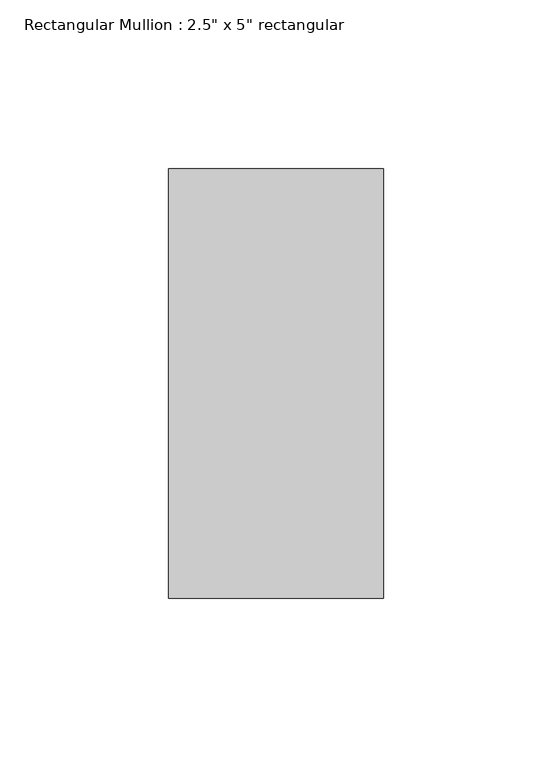
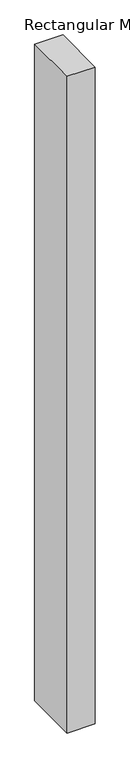
"""IFC4 building model written with IfcOpenShell, lengths in millimetres: member geometry."""

from ifc_helpers import new_model, si_unit, frame, origin, place, context, project, spatial, polyline, outline, extrude, source, transform, mapped, element, save


def member_e7b97c4b(model_context):
    return source(origin(), model_context, "Body", "SweptSolid", [
        extrude(outline(polyline([(0.0, 63.5), (0.0, -63.5), (-63.5, -63.5), (-63.5, 63.5), (0.0, 63.5)])), frame((0.0, 0.0, -1569.0265415), z_axis=(0.0, 0.0, 1.0), x_axis=(1.0, 0.0, 0.0)), (0.0, 0.0, 1.0), 1569.0265415),
    ])


if __name__ == "__main__":
    model = new_model("IFC4")
    model_context = context("Model", 3, world=origin())
    ifc_project = project(units=[si_unit("LENGTHUNIT", "METRE", prefix="MILLI")], contexts=[model_context])
    site = spatial("IfcSite", under=ifc_project)
    building = spatial("IfcBuilding", under=site)
    placement = place(None, origin())
    member_shape = member_e7b97c4b(model_context)
    element("IfcMember", 1, ObjectType="Rectangular Mullion : 2.5\" x 5\" rectangular", at=placement, inside=building, context=model_context, shape_type="MappedRepresentation", body=[
        mapped(member_shape, transform((0.0, 0.0, 0.0), x_axis=(1.0, 0.0, 0.0), y_axis=(0.0, 1.0, 0.0), z_axis=(0.0, 0.0, 1.0))),
    ])
    save(model, "model.ifc")

# Revit data of these elements
# Type "Rectangular Mullion : 2.5\" x 5\" rectangular"
#   built-in parameter 1007304 = 0.416667 (stored number, unit not read)
#   built-in parameter 1007301 = 0.104167 (stored number, unit not read)
#   built-in parameter 1007300 = 0.104167 (stored number, unit not read)
# Element 1 (IfcMember, "Rectangular Mullion : 2.5\" x 5\" rectangular")
#   Materials on its faces: "Aluminum"
# Materials
#   "Aluminum": class "Metal", colour RGB 247 247 247, transparency 0, Description = "Aluminum 6061", Cost = 0
